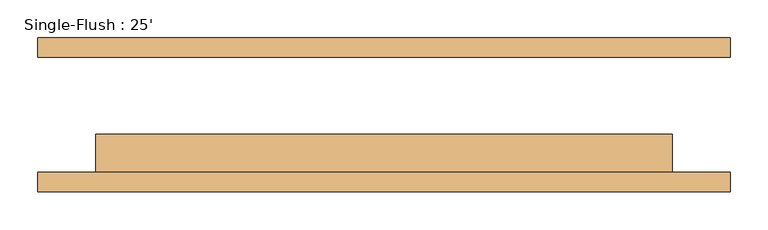
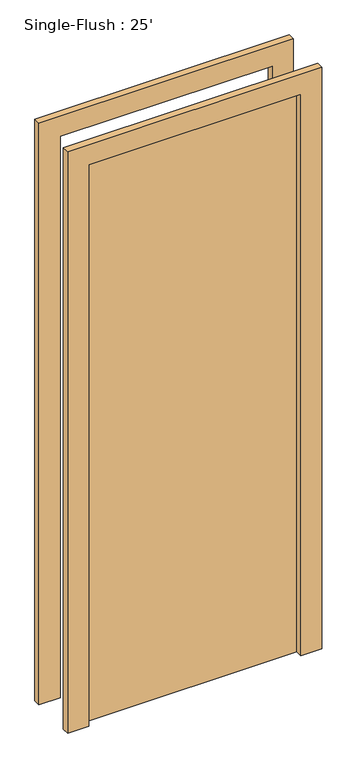
"""IFC4 building model written with IfcOpenShell, lengths in millimetres: door geometry, Single-Flush : 25'."""

from ifc_helpers import new_model, si_unit, frame, origin, origin_with_axes, place, context, project, spatial, polyline, outline, extrude, source, transform, mapped, element, save


def single_flush_25_e2b13fe9(model_context):
    return source(origin(), model_context, "Body", "SweptSolid", [
        extrude(outline(polyline([(2209.8, -457.2), (0.0, -457.2), (0.0, -381.0), (2133.6, -381.0), (2133.6, 381.0), (0.0, 381.0), (0.0, 457.2), (2209.8, 457.2), (2209.8, -457.2)])), frame((0.0, -101.6, 0.0), z_axis=(0.0, 1.0, 0.0), x_axis=(0.0, 0.0, 1.0)), (0.0, 0.0, 1.0), 25.4),
        extrude(outline(polyline([(2209.8, 457.2), (2209.8, -457.2), (0.0, -457.2), (0.0, -381.0), (2133.6, -381.0), (2133.6, 381.0), (0.0, 381.0), (0.0, 457.2), (2209.8, 457.2)])), frame((0.0, 76.2, 0.0), z_axis=(0.0, 1.0, 0.0), x_axis=(0.0, 0.0, 1.0)), (0.0, 0.0, 1.0), 25.4),
        extrude(outline(polyline([(381.0, -25.4), (381.0, -76.2), (-381.0, -76.2), (-381.0, -25.4), (381.0, -25.4)])), origin_with_axes(), (0.0, 0.0, 1.0), 2133.6),
    ])


if __name__ == "__main__":
    model = new_model("IFC4")
    model_context = context("Model", 3, world=origin())
    ifc_project = project(units=[si_unit("LENGTHUNIT", "METRE", prefix="MILLI")], contexts=[model_context])
    site = spatial("IfcSite", under=ifc_project)
    building = spatial("IfcBuilding", under=site)
    placement = place(None, origin())
    single_flush_25_shape = single_flush_25_e2b13fe9(model_context)
    element("IfcDoor", 1, ObjectType="Single-Flush : 25'", at=placement, inside=building, context=model_context, shape_type="MappedRepresentation", body=[
        mapped(single_flush_25_shape, transform((0.0, 0.0, 0.0), x_axis=(1.0, 0.0, 0.0), y_axis=(0.0, 1.0, 0.0), z_axis=(0.0, 0.0, 1.0))),
    ])
    save(model, "model.ifc")

# Revit data of these elements
# Type "Single-Flush : 25'"
#   Type Mark = "8"
#   Construction Type Id = "MDOOR"
#   Assembly Code = "C1020"
#   Analytic Construction = "Metal"
#   Thickness = 0' - 2"
#   Heat Transfer Coefficient (U) = 0.651978 BTU/(h·ft²·°F)
#   Height = 7' - 0"
#   Trim Projection Ext = 0' - 1"
#   Trim Projection Int = 0' - 1"
#   Trim Width = 0' - 3"
#   Width = 2' - 6"
#   Define Thermal Properties by = 1
#   Door Material = Door - Panel
#   Frame Material = Door - Frame
#   Visual Light Transmittance = 0
#   Solar Heat Gain Coefficient = 0
#   Function = (empty or 0)
#   Wall Closure = (empty or 0)
# Element 1 (IfcDoor, "Single-Flush : 25'")
#   Materials on its faces: "Door - Frame", "Door - Panel"
# Materials
#   "Door - Panel": class "Wood", colour RGB 210 159 95, transparency 0
#   "Door - Frame": colour RGB 118 70 51, transparency 0
